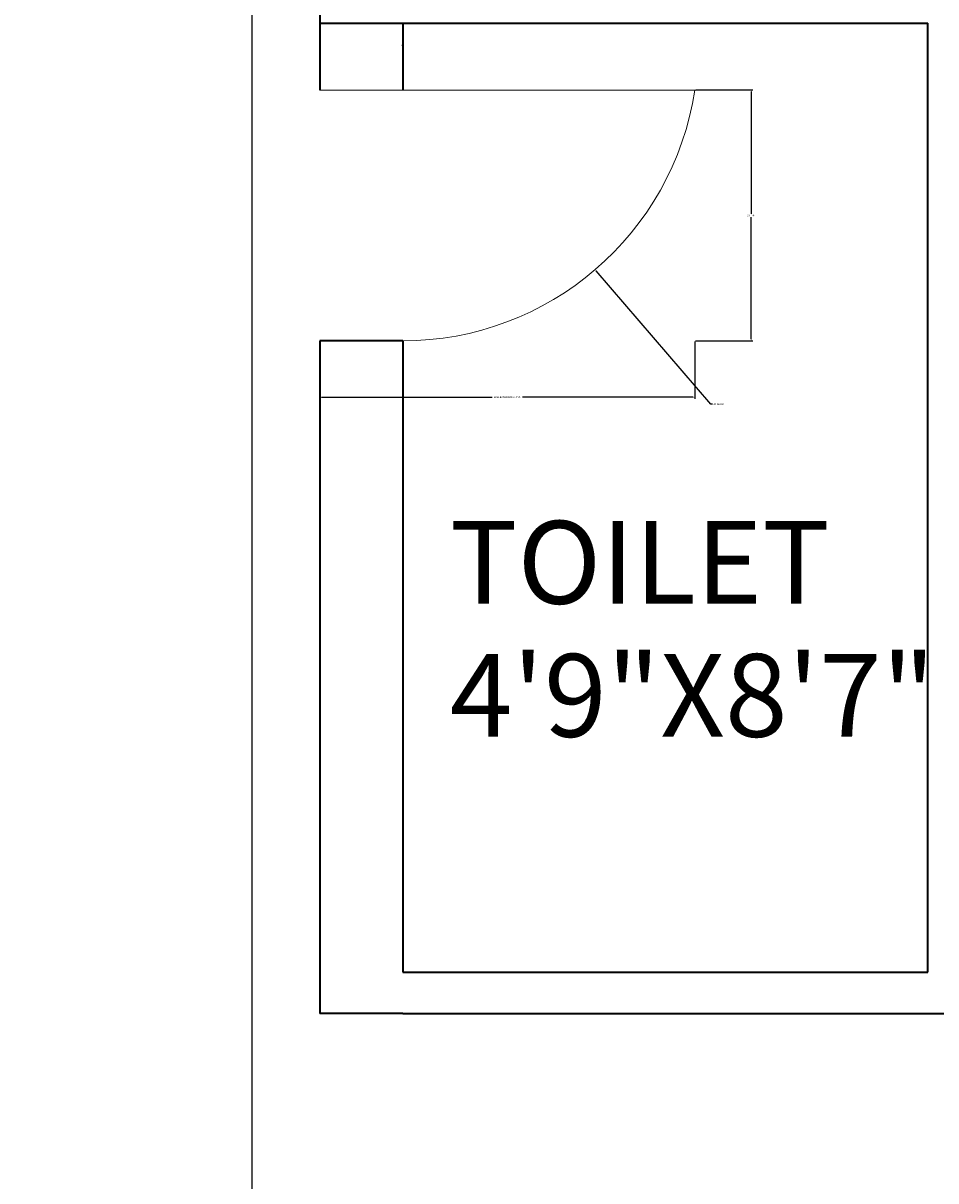
# Model space of a CAD drawing. Units: feet. Extents: x 5816 to 6644, y 25475 to 26788.
# Tile 15 of 23: x 6082 to 6181, y 26373 to 26499. Entities that reach past the tile are written whole.
import ezdxf

# ---------------------------------------------------------------- set-up
doc = ezdxf.new("R2010")
doc.units = ezdxf.units.FT
for name, color, linetype, lineweight in [('A-ANNO-DIMS', 2, 'Continuous', 13), ('A-AREA-IDEN', 7, 'Continuous', 18), ('A-DOOR', 3, 'Continuous', 18), ('A-WALL', 7, 'Continuous', 35)]:
    doc.layers.add(name, color=color, linetype=linetype, lineweight=lineweight)
doc.styles.get("Standard").update_dxf_attribs({"font": 'arial.ttf'})
doc.dimstyles.get("Standard").update_dxf_attribs({"dimtxt": 0.18, "dimasz": 0.18, "dimexe": 0.18, "dimexo": 0.0625, "dimgap": 0.09, "dimtad": 0, "dimtih": 1, "dimtoh": 1, "dimdec": 4, "dimzin": 0, "dimdsep": 46, "dimtxsty": 'Standard', "dimcen": 0.09, "dimadec": 0, "dimazin": 0, "dimtfac": 1, "dimtdec": 4, "dimtofl": 0, "dimtmove": 0, "dimatfit": 3, "dimfxl": 1, "dimtolj": 1, "dimtzin": 0, "dimarcsym": 0})

# ---------------------------------------------------------------- blocks, each defined once
blk = doc.blocks.new('DOOR-BATH-HALL')
blk.add_line((40.72, 0), (0, 0))
blk.add_arc((9, 4.86), 32.09, 270, 351.2882)
blk = doc.blocks.new('*D35')
at = {"layer": 'A-ANNO-DIMS', "color": 0, "lineweight": -2, "transparency": 16777216}
for p, q in [((6114.31, 26464.04), (6114.31, 26457.81)), ((6155.03, 26464.04), (6155.03, 26457.81)), ((6114.49, 26457.99), (6133.02, 26457.99)), ((6154.85, 26457.99), (6136.33, 26457.99))]:
    blk.add_line(p, q, dxfattribs=at)
at = {"layer": 'A-ANNO-DIMS', "color": 0, "transparency": 16777216}
for points in [[(6114.49, 26458.02), (6114.49, 26457.96), (6114.31, 26457.99)], [(6154.85, 26458.02), (6154.85, 26457.96), (6155.03, 26457.99)]]:
    blk.add_solid(points, dxfattribs=at)
at = {"layer": 'Defpoints', "color": 0, "transparency": 16777216}
for p in [(6114.31, 26464.1), (6155.03, 26464.1), (6155.03, 26457.99)]:
    blk.add_point(p, dxfattribs=at)
at = {"layer": 'A-ANNO-DIMS', "color": 0, "transparency": 16777216, "insert": (6134.67, 26457.99), "char_height": 0.18, "attachment_point": 5}
blk.add_mtext('\\A1;HALL BATH DOOR 41 TYP.', dxfattribs=at)
blk = doc.blocks.new('*D36')
at = {"layer": 'A-ANNO-DIMS', "color": 0, "lineweight": -2, "transparency": 16777216}
for p, q in [((6155.1, 26491.33), (6161.32, 26491.33)), ((6161.14, 26491.15), (6161.14, 26477.89)), ((6161.14, 26464.28), (6161.14, 26477.53)), ((6155.1, 26464.1), (6161.32, 26464.1))]:
    blk.add_line(p, q, dxfattribs=at)
at = {"layer": 'A-ANNO-DIMS', "color": 0, "transparency": 16777216}
for points in [[(6161.11, 26491.15), (6161.17, 26491.15), (6161.14, 26491.33)], [(6161.11, 26464.28), (6161.17, 26464.28), (6161.14, 26464.1)]]:
    blk.add_solid(points, dxfattribs=at)
at = {"layer": 'Defpoints', "color": 0, "transparency": 16777216}
for p in [(6155.03, 26491.33), (6161.14, 26491.33), (6155.03, 26464.1)]:
    blk.add_point(p, dxfattribs=at)
at = {"layer": 'A-ANNO-DIMS', "color": 0, "transparency": 16777216, "insert": (6161.14, 26477.71), "char_height": 0.18, "attachment_point": 5}
blk.add_mtext('\\A1;27 TYP.', dxfattribs=at)
blk = doc.blocks.new('*D58')
at = {"layer": 'A-ANNO-DIMS', "color": 0, "lineweight": -2, "transparency": 16777216}
for p, q in [((5953.98, 26168.65), (5953.98, 26787.91)), ((5954.16, 26787.73), (6030.2, 26787.73)), ((6106.8, 26787.73), (6030.76, 26787.73)), ((6106.98, 26168.71), (6106.98, 26787.91))]:
    blk.add_line(p, q, dxfattribs=at)
at = {"layer": 'A-ANNO-DIMS', "color": 0, "transparency": 16777216}
for points in [[(5954.16, 26787.76), (5954.16, 26787.7), (5953.98, 26787.73)], [(6106.8, 26787.76), (6106.8, 26787.7), (6106.98, 26787.73)]]:
    blk.add_solid(points, dxfattribs=at)
at = {"layer": 'Defpoints', "color": 0, "transparency": 16777216}
for p in [(6106.98, 26787.73), (5953.98, 26168.58), (6106.98, 26168.65)]:
    blk.add_point(p, dxfattribs=at)
at = {"layer": 'A-ANNO-DIMS', "color": 0, "transparency": 16777216, "insert": (6030.48, 26787.73), "char_height": 0.18, "attachment_point": 5}
blk.add_mtext('\\A1;153', dxfattribs=at)
blk = doc.blocks.new('*D60')
at = {"layer": 'A-ANNO-DIMS', "color": 0, "lineweight": -2, "transparency": 16777216}
for p, q in [((6106.98, 26094.4), (6106.98, 26787.91)), ((6107.16, 26787.73), (6224.93, 26787.73)), ((6343.5, 26787.73), (6225.72, 26787.73)), ((6343.68, 26094.4), (6343.68, 26787.91))]:
    blk.add_line(p, q, dxfattribs=at)
at = {"layer": 'A-ANNO-DIMS', "color": 0, "transparency": 16777216}
for points in [[(6107.16, 26787.76), (6107.16, 26787.7), (6106.98, 26787.73)], [(6343.5, 26787.76), (6343.5, 26787.7), (6343.68, 26787.73)]]:
    blk.add_solid(points, dxfattribs=at)
at = {"layer": 'Defpoints', "color": 0, "transparency": 16777216}
for p in [(6343.68, 26787.73), (6106.98, 26094.34), (6343.68, 26094.34)]:
    blk.add_point(p, dxfattribs=at)
at = {"layer": 'A-ANNO-DIMS', "color": 0, "transparency": 16777216, "insert": (6225.33, 26787.73), "char_height": 0.18, "attachment_point": 5}
blk.add_mtext('\\A1;236.7', dxfattribs=at)
blk = doc.blocks.new('*D77')
at = {"layer": 'A-ANNO-DIMS', "color": 0, "lineweight": -2, "transparency": 16777216}
for p, q in [((6123.22, 26496.19), (6123.4, 26496.19)), ((6123.31, 26496.1), (6123.31, 26496.28)), ((6156.76, 26457.23), (6144.33, 26471.7)), ((6156.94, 26457.23), (6156.76, 26457.23))]:
    blk.add_line(p, q, dxfattribs=at)
at = {"layer": 'A-ANNO-DIMS', "color": 0, "transparency": 16777216}
blk.add_solid([(6144.35, 26471.72), (6144.31, 26471.68), (6144.21, 26471.84)], dxfattribs=at)
at = {"layer": 'Defpoints', "color": 0, "transparency": 16777216}
for p in [(6123.31, 26496.19), (6144.21, 26471.84)]:
    blk.add_point(p, dxfattribs=at)
at = {"layer": 'A-ANNO-DIMS', "color": 0, "transparency": 16777216, "insert": (6157.61, 26457.23), "char_height": 0.18, "attachment_point": 5}
blk.add_mtext('\\A1;4X R32.09', dxfattribs=at)

msp = doc.modelspace()

# ---------------------------------------------------------------- linework, layer by layer
at = {"layer": 'A-WALL'}
for p, q in [((6114.3119, 26558.5846), (6114.3119, 26491.3288)), ((6114.3119, 26498.5846), (6180.3119, 26498.5846)), ((6123.3119, 26498.5846), (6123.3119, 26491.3288)), ((6180.3119, 26395.5846), (6180.3119, 26498.5846)), ((6123.3119, 26464.0978), (6114.3119, 26464.0978)), ((6114.3119, 26464.0978), (6114.3119, 26391.0846)), ((6123.3119, 26464.0978), (6123.3119, 26395.5846)), ((6123.3119, 26395.5846), (6180.3119, 26395.5846)), ((6123.3119, 26391.0846), (6114.3119, 26391.0846)), ((6123.3119, 26391.0846), (6225.3119, 26391.0846))]:
    msp.add_line(p, q, dxfattribs=at)

# ---------------------------------------------------------------- block references
at = {"layer": 'A-DOOR'}
msp.add_blockref('DOOR-BATH-HALL', (6114.3119, 26491.3288), dxfattribs=at)

# ---------------------------------------------------------------- texts
at = {"layer": 'A-ANNO-DIMS'}
msp.add_text('4\'9"X8\'7"', height=8.98988, dxfattribs=at).set_placement((6128.4298, 26421.1254))
at = {"layer": 'A-AREA-IDEN'}
msp.add_text('TOILET', height=8.98988, dxfattribs=at).set_placement((6128.4298, 26435.5669))

# ---------------------------------------------------------------- dimensions: what is measured, and where the dimension line sits
at = {"layer": 'A-ANNO-DIMS'}
for base, p1, p2, override, picture, middle in [((6106.9781, 26787.7346), (5953.9781, 26168.5846), (6106.9781, 26168.6509), {"dimdec": 0, "dimlfac": 1, "dimrnd": 0, "dimzin": 0, "dimdsep": 46, "dimlunit": 2}, '*D58', (6030.4781, 26787.7346)), ((6343.6763, 26787.7346), (6106.9781, 26094.3368), (6343.6763, 26094.3368), {"dimdec": 1, "dimlfac": 1, "dimrnd": 0, "dimzin": 0, "dimdsep": 46, "dimlunit": 2}, '*D60', (6225.3272, 26787.7346))]:
    dim = msp.add_linear_dim(base=base, p1=p1, p2=p2, dimstyle='Standard', override=override, dxfattribs=at)
    dim.commit()
    dim.dimension.update_dxf_attribs({"geometry": picture, "text_midpoint": middle})
dim = msp.add_radius_dim(center=(6123.3119, 26496.1895), mpoint=(6144.2149, 26471.8391), text='4X <>', dimstyle='Standard', override={"dimdec": 2, "dimlfac": 1, "dimrnd": 0, "dimzin": 0, "dimdsep": 46, "dimlunit": 2}, dxfattribs=at)
dim.commit()
dim.dimension.update_dxf_attribs({"geometry": '*D77', "text_midpoint": (6157.6137, 26457.2289), "dimtype": 164})
dim = msp.add_linear_dim(base=(6161.1415, 26491.3288), p1=(6155.0333, 26464.0978), p2=(6155.0333, 26491.3288), angle=90, text='<> TYP.', dimstyle='Standard', override={"dimdec": 0, "dimlfac": 1, "dimrnd": 0, "dimzin": 0, "dimdsep": 46, "dimlunit": 2}, dxfattribs=at)
dim.commit()
dim.dimension.update_dxf_attribs({"geometry": '*D36', "text_midpoint": (6161.1415, 26477.7133)})
dim = msp.add_linear_dim(base=(6155.0333, 26457.9896), p1=(6114.3119, 26464.0978), p2=(6155.0333, 26464.0978), text='HALL BATH DOOR <> TYP.', dimstyle='Standard', override={"dimdec": 0, "dimlfac": 1, "dimrnd": 0, "dimzin": 0, "dimdsep": 46, "dimlunit": 2}, dxfattribs=at)
dim.commit()
dim.dimension.update_dxf_attribs({"geometry": '*D35', "text_midpoint": (6134.6726, 26457.9896)})

doc.saveas('drawing.dxf')
